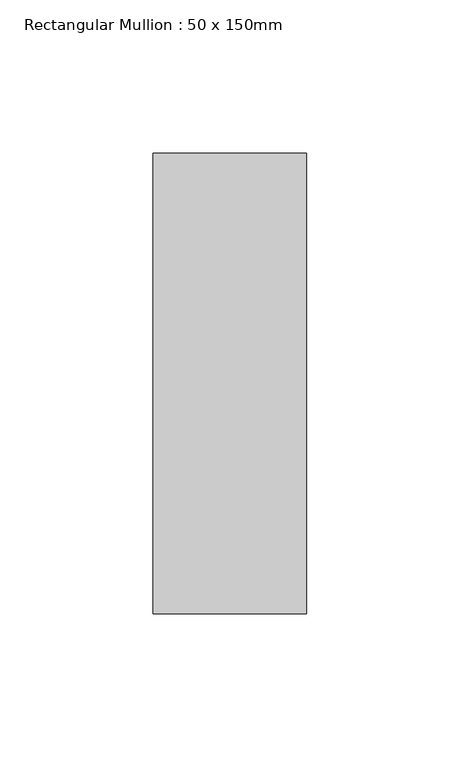
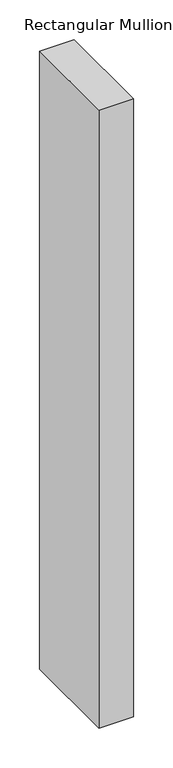
"""IFC4 building model written with IfcOpenShell, lengths in millimetres: member geometry, Rectangular Mullion : 50 x 150mm."""

from ifc_helpers import new_model, si_unit, frame, origin, place, context, project, spatial, polyline, outline, extrude, source, transform, mapped, element, save


def rectangular_mullion_50_x_150mm_2615a836(model_context):
    return source(origin(), model_context, "Body", "SweptSolid", [
        extrude(outline(polyline([(25.0, 75.0), (25.0, -75.0), (-25.0, -75.0), (-25.0, 75.0), (25.0, 75.0)])), frame((0.0, 0.0, -950.0000001), z_axis=(0.0, 0.0, 1.0), x_axis=(1.0, 0.0, 0.0)), (0.0, 0.0, 1.0), 950.0000001),
    ])


if __name__ == "__main__":
    model = new_model("IFC4")
    model_context = context("Model", 3, world=origin())
    ifc_project = project(units=[si_unit("LENGTHUNIT", "METRE", prefix="MILLI")], contexts=[model_context])
    site = spatial("IfcSite", under=ifc_project)
    building = spatial("IfcBuilding", under=site)
    placement = place(None, origin())
    rectangular_mullion_50_x_150mm_shape = rectangular_mullion_50_x_150mm_2615a836(model_context)
    element("IfcMember", 1, ObjectType="Rectangular Mullion : 50 x 150mm", at=placement, inside=building, context=model_context, shape_type="MappedRepresentation", body=[
        mapped(rectangular_mullion_50_x_150mm_shape, transform((0.0, 0.0, 0.0), x_axis=(1.0, 0.0, 0.0), y_axis=(0.0, 1.0, 0.0), z_axis=(0.0, 0.0, 1.0))),
    ])
    save(model, "model.ifc")

# Revit data of these elements
# Type "Rectangular Mullion : 50 x 150mm"
#   built-in parameter 1007304 = 0.492126 (stored number, unit not read)
#   built-in parameter 1007301 = 0.082021 (stored number, unit not read)
#   built-in parameter 1007300 = 0.082021 (stored number, unit not read)
# Element 1 (IfcMember, "Rectangular Mullion : 50 x 150mm")
#   Materials on its faces: "Aluminium"
# Materials
#   "Aluminium": class "Metal", colour RGB 247 247 247, transparency 0, Description = "Aluminium 6061", Cost = 0
